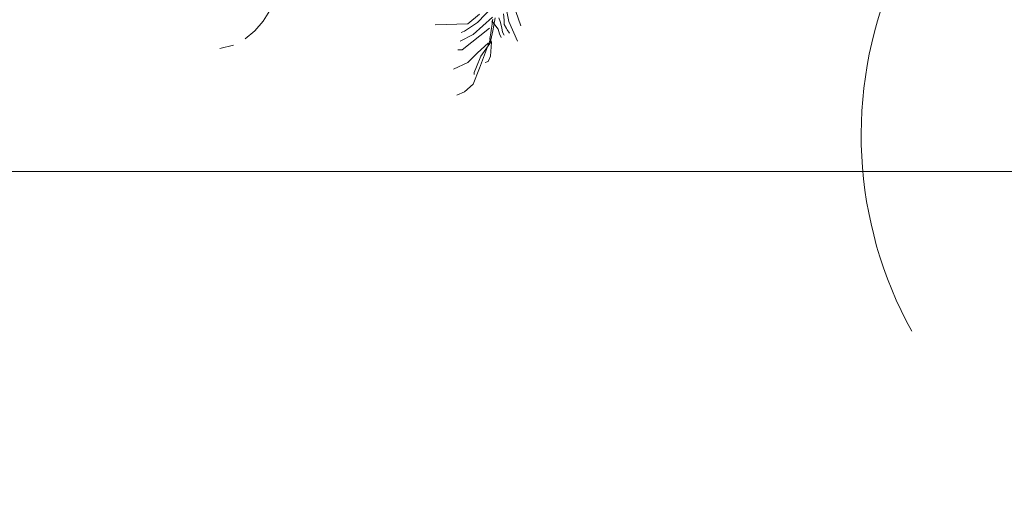
# Model space of a CAD drawing. Units: millimetres. Extents: x 595116 to 630915, y 909473 to 920225.
# Tile 19 of 134: x 629596 to 629622, y 919152 to 919165. Entities that reach past the tile are written whole.
import ezdxf

# ---------------------------------------------------------------- set-up
doc = ezdxf.new("R2010")
doc.units = ezdxf.units.MM
doc.layers.add('Dimension', color=3, linetype='Continuous', lineweight=18)
doc.layers.add('L-PLNT', color=85, linetype='Continuous', lineweight=13)
doc.styles.get("Standard").update_dxf_attribs({"font": 'arial.ttf'})
doc.dimstyles.new('ISO-25', dxfattribs={"dimtxt": 9, "dimasz": 6, "dimexe": 1.25, "dimexo": 0.625, "dimtad": 1, "dimlunit": 4, "dimtxsty": 'Standard', "dimcen": 2.5, "dimadec": 0, "dimazin": 0, "dimtfac": 1, "dimtmove": 0, "dimatfit": 3, "dimfxl": 1, "dimarcsym": 0})

# ---------------------------------------------------------------- blocks, each defined once
blk = doc.blocks.new('tree')
blk.add_arc((629598.153, 919288.998), 5.103, 105.3576, 208.8973)
blk = doc.blocks.new('A$C4FB75ABC')
for p, q in [((3.386, 0.8461), (3.508, 0.4878)), ((3.3708, 0.7927), (3.4242, 0.5183)), ((3.3174, 0.6327), (3.203, 0.5107)), ((1.74, 0.5958), (1.6917, 0.5207)), ((3.2182, 0.5717), (3.1344, 0.5031)), ((3.3855, 0.5721), (3.3909, 0.5291)), ((1.6917, 0.5207), (1.6336, 0.4527)), ((3.1344, 0.5031), (2.9056, 0.4955)), ((3.203, 0.5107), (3.1115, 0.4497)), ((3.3098, 0.5488), (3.1725, 0.4269)), ((3.3034, 0.4863), (3.3013, 0.4707)), ((3.3055, 0.5008), (3.3034, 0.4863)), ((3.3047, 0.5237), (3.3478, 0.4645)), ((3.3075, 0.5137), (3.3055, 0.5008)), ((3.3093, 0.5249), (3.3075, 0.5137)), ((3.3111, 0.5347), (3.3093, 0.5249)), ((3.3282, 0.5451), (3.3124, 0.4531)), ((3.3532, 0.5452), (3.364, 0.5183)), ((3.364, 0.5183), (3.3747, 0.4753)), ((3.3909, 0.5291), (3.3909, 0.4968)), ((3.3909, 0.4968), (3.407, 0.4699)), ((3.4242, 0.5183), (3.4852, 0.3811)), ((1.6336, 0.4527), (1.5642, 0.3956)), ((3.1725, 0.4269), (3.081, 0.3811)), ((3.1115, 0.4497), (3.0886, 0.4421)), ((3.2869, 0.4726), (3.0962, 0.3201)), ((3.3124, 0.4531), (3.2923, 0.3674)), ((3.2949, 0.4237), (3.2929, 0.4103)), ((3.297, 0.4387), (3.2949, 0.4237)), ((3.2992, 0.4546), (3.297, 0.4387)), ((3.3013, 0.4707), (3.2992, 0.4546)), ((3.3478, 0.4645), (3.3586, 0.4322)), ((3.3586, 0.4322), (3.3693, 0.4053)), ((3.3747, 0.4753), (3.3801, 0.443)), ((3.3801, 0.443), (3.3909, 0.4214)), ((3.407, 0.4699), (3.4124, 0.4591)), ((3.4124, 0.4591), (3.4286, 0.4376)), ((1.4819, 0.3527), (1.3853, 0.3277)), ((3.2793, 0.3659), (3.203, 0.2973)), ((3.2945, 0.3964), (3.2182, 0.1906)), ((3.3021, 0.3811), (3.2259, 0.2744)), ((3.2911, 0.3992), (3.2894, 0.3911)), ((3.2929, 0.4103), (3.2911, 0.3992)), ((3.3021, 0.3735), (3.2945, 0.2744)), ((3.0962, 0.3201), (3.0657, 0.3201)), ((3.203, 0.2973), (3.1344, 0.2287)), ((3.1344, 0.2287), (3.0352, 0.1829)), ((3.2259, 0.2744), (3.1954, 0.1982)), ((3.2793, 0.2363), (3.2564, 0.2287)), ((3.2945, 0.2744), (3.2793, 0.2363)), ((3.2182, 0.1906), (3.1725, 0.0762)), ((3.1954, 0.1982), (3.1801, 0.1601)), ((3.1801, 0.1601), (3.1801, 0.1448)), ((3.1725, 0.0762), (3.1115, 0.0229)), ((3.1115, 0.0229), (3.0581, 0))]:
    blk.add_line(p, q)
blk = doc.blocks.new('*D216')
at = {"layer": 'Defpoints', "color": 0, "transparency": 16777216}
for p in [(629743.541, 919411.928), (629505.041, 919411.828), (629743.541, 918832.378)]:
    blk.add_point(p, dxfattribs=at)
at = {"layer": 'Dimension', "color": 0, "lineweight": -2, "transparency": 16777216}
for p, q in [((629505.041, 919411.203), (629505.041, 918831.128)), ((629743.541, 919411.303), (629743.541, 918831.128)), ((629511.041, 918832.378), (629737.541, 918832.378))]:
    blk.add_line(p, q, dxfattribs=at)
at = {"layer": 'Dimension', "color": 0, "transparency": 16777216}
for points in [[(629511.041, 918833.378), (629511.041, 918831.378), (629505.041, 918832.378)], [(629737.541, 918833.378), (629737.541, 918831.378), (629743.541, 918832.378)]]:
    blk.add_solid(points, dxfattribs=at)
at = {"layer": 'Dimension', "color": 0, "transparency": 16777216, "insert": (629624.291, 918837.656), "char_height": 9, "attachment_point": 5}
blk.add_mtext('19\'-10 1/2"', dxfattribs=at)

msp = doc.modelspace()

# ---------------------------------------------------------------- linework, layer by layer
at = {"layer": 'L-PLNT'}
msp.add_line((629511.274, 919160.917), (629824.951, 919160.917), dxfattribs=at)

# ---------------------------------------------------------------- block references
for name, p, xscale, yscale, zscale in [('tree', (-697368.484, -1018413.796), 2.107689410566463, 2.107689410566463, 2.107689410566463), ('A$C4FB75ABC', (629595.944, 919162.946), 3.753413438031968, 3.753413438031968, 3.753413438031968)]:
    msp.add_blockref(name, p, dxfattribs=dict(at, xscale=xscale, yscale=yscale, zscale=zscale))

# ---------------------------------------------------------------- dimensions: what is measured, and where the dimension line sits
at = {"layer": 'Dimension'}
dim = msp.add_linear_dim(base=(629743.541, 918832.378), p1=(629505.041, 919411.828), p2=(629743.541, 919411.928), dimstyle='ISO-25', override={"dimdec": 1, "dimlfac": 1, "dimrnd": 0, "dimzin": 1, "dimdsep": 46, "dimlunit": 4, "dimfrac": 2}, dxfattribs=at)
dim.commit()
dim.dimension.update_dxf_attribs({"geometry": '*D216', "text_midpoint": (629624.291, 918837.656)})

doc.saveas('drawing.dxf')
